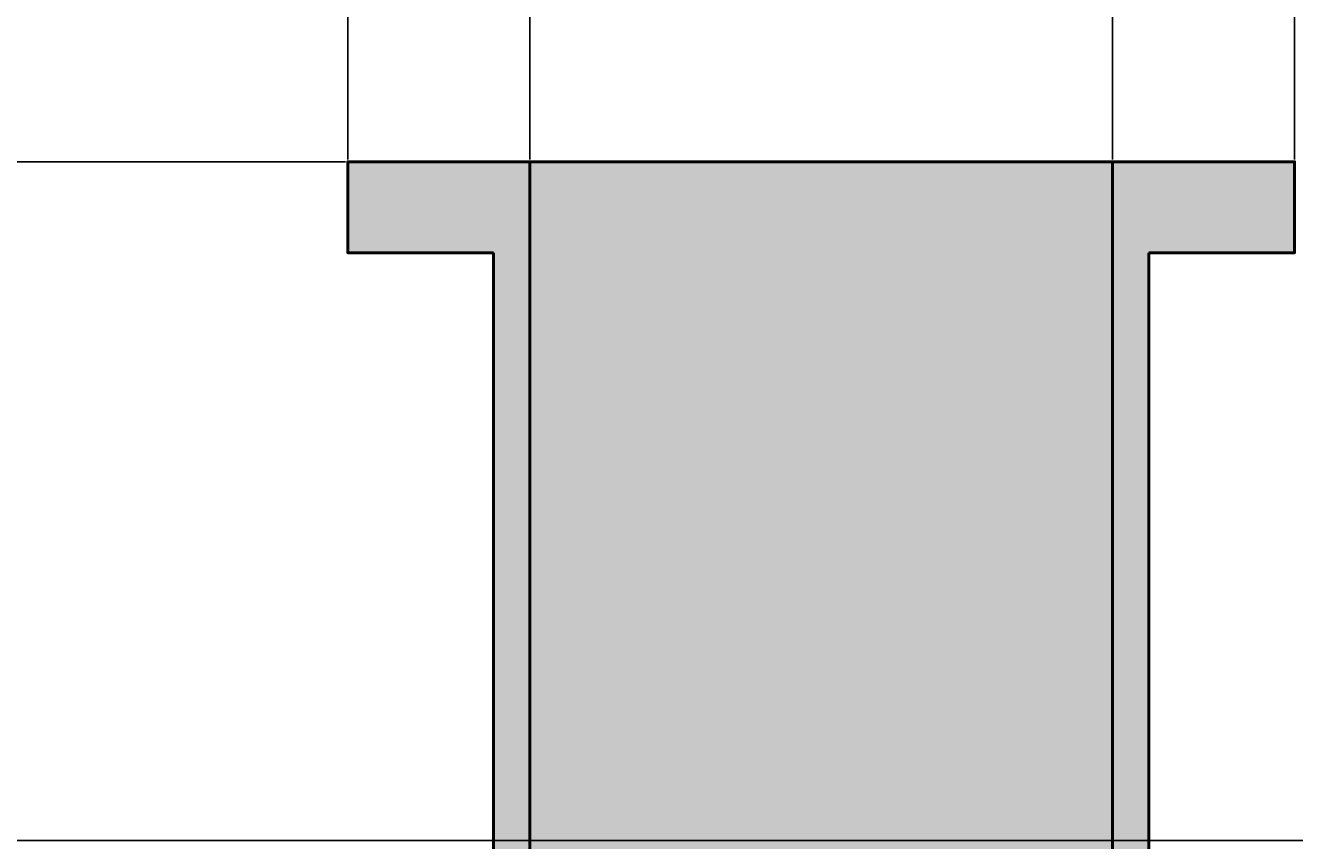
# Model space of a CAD drawing. Units: inches. Extents: x -12 to 334, y -10 to 186.
# Tile 21 of 77: x 23 to 58, y 109 to 131. Entities that reach past the tile are written whole.
import ezdxf

# ---------------------------------------------------------------- set-up
doc = ezdxf.new("R2010")
doc.units = ezdxf.units.IN
doc.header["$MEASUREMENT"] = 0
for name, color, linetype, lineweight in [('M-DIMS', 2, 'Continuous', 18), ('M-EQPM', 7, 'Continuous', 50), ('M-EQPM-PATT', 8, 'Continuous', 18)]:
    doc.layers.add(name, color=color, linetype=linetype, lineweight=lineweight)
doc.styles.get("Standard").update_dxf_attribs({"font": 'arial.ttf'})
doc.dimstyles.get("Standard").update_dxf_attribs({"dimtxt": 0.18, "dimasz": 0.18, "dimexe": 0.18, "dimexo": 0.0625, "dimgap": 0.09, "dimtad": 0, "dimtih": 1, "dimtoh": 1, "dimdec": 4, "dimzin": 0, "dimdsep": 46, "dimtxsty": 'Standard', "dimcen": 0.09, "dimadec": 0, "dimazin": 0, "dimtfac": 1, "dimtdec": 4, "dimtofl": 0, "dimtmove": 0, "dimatfit": 3, "dimfxl": 1, "dimtolj": 1, "dimtzin": 0, "dimarcsym": 0})

# ---------------------------------------------------------------- blocks, each defined once
blk = doc.blocks.new('*D2')
at = {"layer": 'Defpoints', "color": 0, "transparency": 16777216}
for p in [(32.1, 169.385), (32.1, 127.708), (3.376, 80.692)]:
    blk.add_point(p, dxfattribs=at)
at = {"layer": 'M-DIMS', "color": 0, "lineweight": -2, "transparency": 16777216}
for p, q in [((3.376, 80.754), (3.376, 169.565)), ((32.1, 127.77), (32.1, 169.565)), ((3.556, 169.385), (17.274, 169.385)), ((31.92, 169.385), (18.203, 169.385))]:
    blk.add_line(p, q, dxfattribs=at)
at = {"layer": 'M-DIMS', "color": 0, "transparency": 16777216}
for points in [[(3.556, 169.415), (3.556, 169.355), (3.376, 169.385)], [(31.92, 169.415), (31.92, 169.355), (32.1, 169.385)]]:
    blk.add_solid(points, dxfattribs=at)
at = {"layer": 'M-DIMS', "color": 0, "transparency": 16777216, "insert": (17.738, 169.385), "char_height": 0.18, "attachment_point": 5}
blk.add_mtext('\\A1;28.724', dxfattribs=at)
blk = doc.blocks.new('*D3')
at = {"layer": 'Defpoints', "color": 0, "transparency": 16777216}
for p in [(58.1, 169.385), (32.1, 127.708), (58.1, 127.708)]:
    blk.add_point(p, dxfattribs=at)
at = {"layer": 'M-DIMS', "color": 0, "lineweight": -2, "transparency": 16777216}
for p, q in [((32.1, 127.77), (32.1, 169.565)), ((58.1, 127.77), (58.1, 169.565)), ((32.28, 169.385), (44.88, 169.385)), ((57.92, 169.385), (45.321, 169.385))]:
    blk.add_line(p, q, dxfattribs=at)
at = {"layer": 'M-DIMS', "color": 0, "transparency": 16777216}
for points in [[(32.28, 169.415), (32.28, 169.355), (32.1, 169.385)], [(57.92, 169.415), (57.92, 169.355), (58.1, 169.385)]]:
    blk.add_solid(points, dxfattribs=at)
at = {"layer": 'M-DIMS', "color": 0, "transparency": 16777216, "insert": (45.1, 169.385), "char_height": 0.18, "attachment_point": 5}
blk.add_mtext('\\A1;26', dxfattribs=at)
blk = doc.blocks.new('*D4')
at = {"layer": 'Defpoints', "color": 0, "transparency": 16777216}
for p in [(53.1, 169.385), (37.1, 127.708), (53.1, 127.708)]:
    blk.add_point(p, dxfattribs=at)
at = {"layer": 'M-DIMS', "color": 0, "lineweight": -2, "transparency": 16777216}
for p, q in [((37.1, 127.77), (37.1, 169.565)), ((53.1, 127.77), (53.1, 169.565)), ((37.28, 169.385), (44.89, 169.385)), ((52.92, 169.385), (45.311, 169.385))]:
    blk.add_line(p, q, dxfattribs=at)
at = {"layer": 'M-DIMS', "color": 0, "transparency": 16777216}
for points in [[(37.28, 169.415), (37.28, 169.355), (37.1, 169.385)], [(52.92, 169.415), (52.92, 169.355), (53.1, 169.385)]]:
    blk.add_solid(points, dxfattribs=at)
at = {"layer": 'M-DIMS', "color": 0, "transparency": 16777216, "insert": (45.1, 169.385), "char_height": 0.18, "attachment_point": 5}
blk.add_mtext('\\A1;16', dxfattribs=at)
blk = doc.blocks.new('*D8')
at = {"layer": 'Defpoints', "color": 0, "transparency": 16777216}
for p in [(-11.174, 127.708), (32.1, 127.708), (23.581, 100.896)]:
    blk.add_point(p, dxfattribs=at)
at = {"layer": 'M-DIMS', "color": 0, "lineweight": -2, "transparency": 16777216}
for p, q in [((32.038, 127.708), (-11.354, 127.708)), ((-11.174, 127.528), (-11.174, 114.484)), ((-11.174, 101.076), (-11.174, 114.12)), ((23.518, 100.896), (-11.354, 100.896))]:
    blk.add_line(p, q, dxfattribs=at)
at = {"layer": 'M-DIMS', "color": 0, "transparency": 16777216}
for points in [[(-11.204, 127.528), (-11.144, 127.528), (-11.174, 127.708)], [(-11.204, 101.076), (-11.144, 101.076), (-11.174, 100.896)]]:
    blk.add_solid(points, dxfattribs=at)
at = {"layer": 'M-DIMS', "color": 0, "transparency": 16777216, "insert": (-11.174, 114.302), "char_height": 0.18, "attachment_point": 5}
blk.add_mtext('\\A1;26.81', dxfattribs=at)
blk = doc.blocks.new('*D14')
at = {"layer": 'Defpoints', "color": 0, "transparency": 16777216}
for p in [(63.5, 109.058), (-11.174, 49.45), (64.207, 49.45)]:
    blk.add_point(p, dxfattribs=at)
at = {"layer": 'M-DIMS', "color": 0, "lineweight": -2, "transparency": 16777216}
for p, q in [((63.438, 109.058), (-11.354, 109.058)), ((-11.174, 108.878), (-11.174, 79.436)), ((-11.174, 49.63), (-11.174, 79.072)), ((64.144, 49.45), (-11.354, 49.45))]:
    blk.add_line(p, q, dxfattribs=at)
at = {"layer": 'M-DIMS', "color": 0, "transparency": 16777216}
for points in [[(-11.204, 108.878), (-11.144, 108.878), (-11.174, 109.058)], [(-11.204, 49.63), (-11.144, 49.63), (-11.174, 49.45)]]:
    blk.add_solid(points, dxfattribs=at)
at = {"layer": 'M-DIMS', "color": 0, "transparency": 16777216, "insert": (-11.174, 79.254), "char_height": 0.18, "attachment_point": 5}
blk.add_mtext('\\A1;59.61', dxfattribs=at)

msp = doc.modelspace()

# ---------------------------------------------------------------- hatches: boundary and pattern name
at = {"layer": 'M-EQPM-PATT'}
h = msp.add_hatch(color=256, dxfattribs=at)
h.set_gradient(color1=(99, 100, 102), color2=(99, 100, 102), tint=1)
h.paths.add_polyline_path([(4.3766, 80.754, -0.4132606), (23.5807, 99.8958), (37.1002, 99.8958), (37.1002, 127.7078), (32.1002, 127.7078), (32.1002, 125.2078), (36.1002, 125.2078), (36.1002, 100.8958), (23.5807, 100.8958, 1), (23.5807, 60.4872), (36.1002, 60.4872), (36.1002, 36.1752), (32.1002, 36.1752), (32.1002, 33.6752), (37.1002, 33.6752), (37.1002, 61.4872), (23.5807, 61.4872, -0.384914), (4.4744, 78.754), (72.9244, 78.754), (72.9244, 69.6117), (75.9244, 69.6117), (75.9244, 89.8963), (72.9244, 89.8963), (72.9244, 80.754)])
h.paths.add_polyline_path([(54.1002, 125.2078), (58.1002, 125.2078), (58.1002, 127.7078), (53.1002, 127.7078), (53.1002, 99.8958), (64.5, 99.8958), (64.5, 109.0583), (63.5, 109.0583), (63.5, 100.8958), (54.1002, 100.8958)], flags=17)
h.paths.add_polyline_path([(53.1002, 33.6752), (58.1002, 33.6752), (58.1002, 36.1752), (54.1002, 36.1752), (54.1002, 60.4872), (64.2068, 60.4872), (64.2068, 49.4497), (87.8879, 49.4497), (87.8879, 55.3205), (104.8919, 55.3205), (104.8919, 30.8541), (99.8919, 30.8541), (99.8919, 28.8541), (105.8919, 28.8541), (105.8919, 56.3205), (87.8879, 56.3205), (87.8879, 63.6117), (86.8879, 63.6117), (86.8879, 50.4497), (65.0061, 50.4497), (65.0061, 63.6117), (64.5, 63.6117), (64.5, 61.4872), (53.1002, 61.4872)])
h.paths.add_polyline_path([(121.8919, 28.8541), (121.8919, 30.8541), (116.8919, 30.8541), (116.8919, 45.8541), (209.6965, 45.8541), (209.9204, 46.8541), (115.8919, 46.8541), (115.8919, 28.8541)])
h.paths.add_polyline_path([(221.5761, 32.8541), (216.5761, 32.8541), (216.5761, 30.8541), (222.5761, 30.8541), (222.5761, 46.8541), (209.9204, 46.8541), (209.6965, 45.8541), (221.5761, 45.8541)])
h.paths.add_polyline_path([(233.5761, 45.8541), (249.8485, 45.8541), (249.3759, 46.8541), (232.5761, 46.8541), (232.5761, 30.8541), (238.5761, 30.8541), (238.5761, 32.8541), (233.5761, 32.8541)])
h = msp.add_hatch(color=256, dxfattribs=at)
h.set_gradient(color1=(205, 32, 39), color2=(205, 32, 39), tint=1)
h.paths.add_polyline_path([(64.5, 80.754), (64.5, 89.8963), (226.6083, 89.8963, -1), (226.6083, 69.6117), (64.5, 69.6117), (64.5, 78.754), (4.4744, 78.754, 0.384914), (23.5807, 61.4872), (37.1002, 61.4872), (37.1002, 33.6752), (53.1002, 33.6752), (53.1002, 61.4872), (64.5, 61.4872), (64.5, 63.6117), (226.6083, 63.6117, 1), (226.6083, 95.8963), (64.5, 95.8963), (64.5, 99.8958), (53.1002, 99.8958), (53.1002, 127.7078), (37.1002, 127.7078), (37.1002, 99.8958), (23.5807, 99.8958, 0.4132606), (4.3766, 80.754)])
h.paths.add_polyline_path([(64.5, 91.8963), (64.5, 93.8963), (226.6083, 93.8963, -1), (226.6083, 65.6117), (64.5, 65.6117), (64.5, 67.6117), (226.6083, 67.6117, 1), (226.6083, 91.8963)], flags=16)

# ---------------------------------------------------------------- linework, layer by layer
at = {"layer": 'M-EQPM'}
for p, q in [((37.1002, 99.8958), (37.1002, 127.7078)), ((53.1002, 99.8958), (53.1002, 127.7078)), ((36.1002, 100.8958), (36.1002, 125.2078)), ((54.1002, 100.8958), (54.1002, 125.2078))]:
    msp.add_line(p, q, dxfattribs=at)
msp.add_lwpolyline([(36.1002, 125.2078), (32.1002, 125.2078), (32.1002, 127.7078), (58.1002, 127.7078), (58.1002, 125.2078), (54.1002, 125.2078)], dxfattribs=at)

# ---------------------------------------------------------------- dimensions: what is measured, and where the dimension line sits
at = {"layer": 'M-DIMS'}
for base, p1, p2, override, picture, middle in [((32.1002, 169.3845), (3.3765, 80.6915), (32.1002, 127.7078), {"dimdec": 3, "dimlfac": 1, "dimrnd": 0, "dimzin": 0, "dimdsep": 46, "dimlunit": 2}, '*D2', (17.7383, 169.3845)), ((58.1002, 169.3845), (32.1002, 127.7078), (58.1002, 127.7078), {"dimdec": 0, "dimlfac": 1, "dimrnd": 0, "dimzin": 0, "dimdsep": 46, "dimlunit": 2}, '*D3', (45.1002, 169.3845)), ((53.1002, 169.3845), (37.1002, 127.7078), (53.1002, 127.7078), {"dimdec": 0, "dimlfac": 1, "dimrnd": 0, "dimzin": 0, "dimdsep": 46, "dimlunit": 2}, '*D4', (45.1002, 169.3845))]:
    dim = msp.add_linear_dim(base=base, p1=p1, p2=p2, dimstyle='Standard', override=override, dxfattribs=at)
    dim.commit()
    dim.dimension.update_dxf_attribs({"geometry": picture, "text_midpoint": middle})
for base, p1, p2, picture, middle in [((-11.1736, 127.7078), (23.5807, 100.8958), (32.1002, 127.7078), '*D8', (-11.1735, 114.3018)), ((-11.1736, 49.4497), (63.5, 109.0583), (64.2068, 49.4497), '*D14', (-11.1735, 79.254))]:
    dim = msp.add_linear_dim(base=base, p1=p1, p2=p2, angle=90, dimstyle='Standard', override={"dimdec": 2, "dimlfac": 1, "dimrnd": 0, "dimzin": 0, "dimdsep": 46, "dimlunit": 2}, dxfattribs=at)
    dim.commit()
    dim.dimension.update_dxf_attribs({"geometry": picture, "text_midpoint": middle})

doc.saveas('drawing.dxf')
